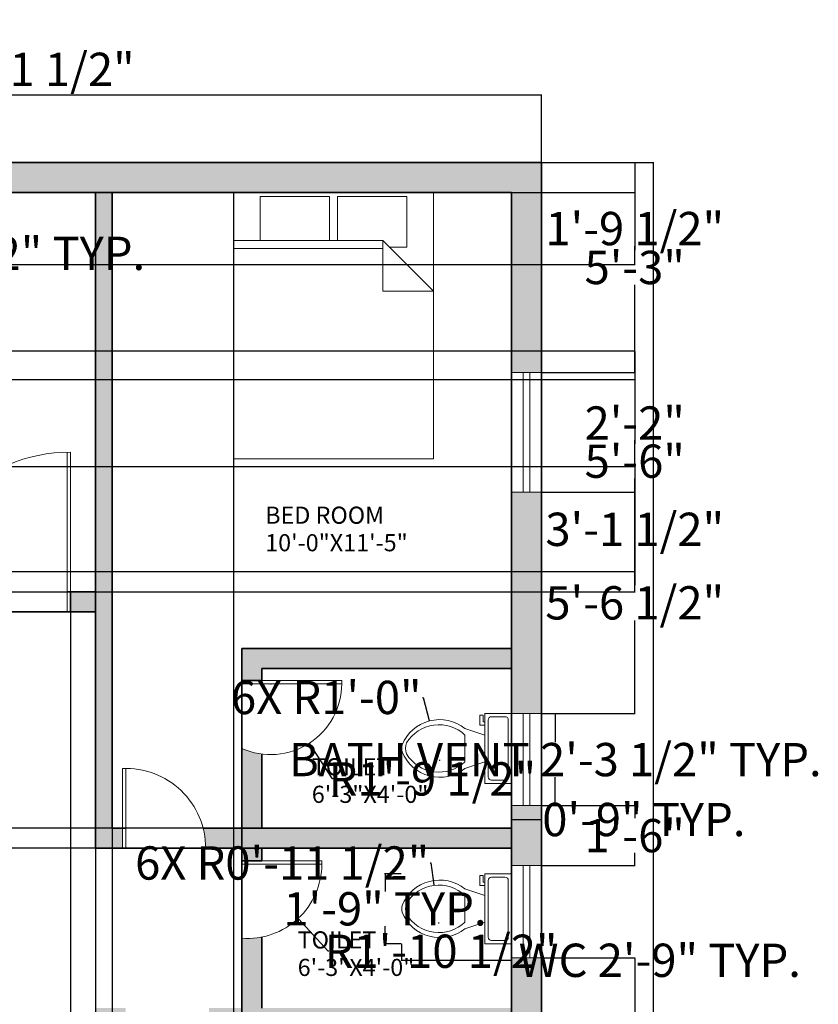
# Model space of a CAD drawing. Units: inches. Extents: x 2172 to 2712, y 1494 to 2108.
# Tile 3 of 3: x 2422 to 2662, y 1812 to 2108. Entities that reach past the tile are written whole.
import ezdxf

# ---------------------------------------------------------------- set-up
doc = ezdxf.new("R2010")
doc.units = ezdxf.units.IN
doc.header["$MEASUREMENT"] = 0
for name, color, linetype, lineweight in [('A-ANNO-DIMS', 2, 'Continuous', 18), ('A-AREA-IDEN', 7, 'Continuous', 18), ('A-DOOR', 3, 'Continuous', 18), ('A-FLOR-FIXT', 9, 'Continuous', 18), ('A-FURN', 8, 'Continuous', 18), ('A-GLAZ', 4, 'Continuous', 18), ('A-WALL', 7, 'Continuous', 35)]:
    doc.layers.add(name, color=color, linetype=linetype, lineweight=lineweight)
doc.layers.add('A-WALL-PATT', color=251, linetype='Continuous', lineweight=13, true_color=0x636466)
doc.styles.get("Standard").update_dxf_attribs({"font": 'arial.ttf'})
doc.dimstyles.get("Standard").update_dxf_attribs({"dimtxt": 10, "dimasz": 0.18, "dimexe": 0.18, "dimexo": 0.0625, "dimgap": 0.09, "dimtad": 0, "dimtih": 1, "dimtoh": 1, "dimdec": 0, "dimzin": 0, "dimdsep": 46, "dimlunit": 3, "dimtxsty": 'Standard', "dimcen": 0.09, "dimadec": 0, "dimazin": 0, "dimtfac": 1, "dimtdec": 0, "dimtofl": 0, "dimtmove": 0, "dimatfit": 3, "dimfxl": 1, "dimtolj": 1, "dimtzin": 0, "dimarcsym": 0})

# ---------------------------------------------------------------- blocks, each defined once
blk = doc.blocks.new('Toilet - top')
for p, q in [((9.5, -6), (9.5, -2)), ((-10, -8.5), (-8, -8.5)), ((-10, -9.5), (-10, -8.5)), ((-8, -8.5), (-8, -8)), ((-7, -8), (-7, -9.5)), ((-4, -8), (-6, -14)), ((4, -8), (6, -14)), ((-7, -9.5), (-10, -9.5)), ((4, -14), (-4, -14))]:
    blk.add_line(p, q)
blk.add_lwpolyline([(10.5, -8), (10.5, 0), (-10.5, 0), (-10.5, -8)], close=True)
for points in [[(-9.5, -2), (-9.5, -6)], [(8.5, -1), (-8.5, -1)], [(-8.5, -7), (8.5, -7)]]:
    blk.add_lwpolyline(points)
for centre, radius, start, end in [((-8.62, -1.88), 0.884, 81.8699, 188.1301), ((8.62, -1.88), 0.884, 351.8699, 98.1301), ((-8.62, -6.12), 0.884, 171.8699, 278.1301), ((8.62, -6.12), 0.884, 261.8699, 8.1301), ((3.52, -21.58), 12.17, 141.4691, 247.9714), ((4.2, -21.82), 11.33, 136.3677, 238.9468), ((-3.52, -21.58), 12.17, 292.0284, 38.5307), ((-4.2, -21.82), 11.33, 301.053, 43.6321), ((0, -27.88), 4, 245.7318, 294.2682), ((0, -29), 4, 254.8605, 285.1395)]:
    blk.add_arc(centre, radius, start, end)
blk = doc.blocks.new('Bed - Queen')
for p, q in [((0, -80.00003), (0, 0)), ((0, 0), (59.99999, 0)), ((59.99999, 0), (59.99999, -80.00003)), ((7.99999, -1.2), (28.79998, -1.2)), ((7.99999, -14.4), (7.99999, -1.2)), ((28.79998, -1.2), (28.79998, -14.4)), ((31.19999, -1.2), (51.99999, -1.2)), ((31.19999, -14.4), (31.19999, -1.2)), ((51.99999, -1.2), (51.99999, -16.4)), ((0, -14.4), (44.8, -14.4)), ((59.99999, -29.6), (44.8, -14.4)), ((44.8, -14.4), (44.8, -29.6)), ((44.8, -16.8), (0, -16.8)), ((51.99999, -16.4), (46.79936, -16.4)), ((44.8, -29.6), (59.99999, -29.6)), ((59.99999, -80.00003), (0, -80.00003))]:
    blk.add_line(p, q)
blk = doc.blocks.new('*D3')
at = {"layer": 'A-ANNO-DIMS', "color": 0, "lineweight": -2, "transparency": 16777216}
for p, q in [((2230.53, 2064.8), (2230.53, 2085.18)), ((2230.71, 2085), (2395.86, 2085)), ((2578.35, 2085), (2413.19, 2085)), ((2578.53, 2064.8), (2578.53, 2085.18))]:
    blk.add_line(p, q, dxfattribs=at)
at = {"layer": 'A-ANNO-DIMS', "color": 0, "transparency": 16777216}
for points in [[(2230.71, 2085.03), (2230.71, 2084.97), (2230.53, 2085)], [(2578.35, 2085.03), (2578.35, 2084.97), (2578.53, 2085)]]:
    blk.add_solid(points, dxfattribs=at)
at = {"layer": 'Defpoints', "color": 0, "transparency": 16777216}
for p in [(2578.53, 2085), (2230.53, 2064.74), (2578.53, 2064.74)]:
    blk.add_point(p, dxfattribs=at)
at = {"layer": 'A-ANNO-DIMS', "color": 0, "transparency": 16777216, "insert": (2404.53, 2085), "char_height": 10, "attachment_point": 5}
blk.add_mtext("\\A1;29'", dxfattribs=at)
blk = doc.blocks.new('*D4')
at = {"layer": 'A-ANNO-DIMS', "color": 0, "lineweight": -2, "transparency": 16777216}
for p, q in [((2578.59, 2064.74), (2612.28, 2064.74)), ((2612.1, 2064.56), (2612.1, 1805.83)), ((2612.1, 1536.92), (2612.1, 1795.65)), ((2578.59, 1536.74), (2612.28, 1536.74))]:
    blk.add_line(p, q, dxfattribs=at)
at = {"layer": 'A-ANNO-DIMS', "color": 0, "transparency": 16777216}
for points in [[(2612.07, 2064.56), (2612.13, 2064.56), (2612.1, 2064.74)], [(2612.07, 1536.92), (2612.13, 1536.92), (2612.1, 1536.74)]]:
    blk.add_solid(points, dxfattribs=at)
at = {"layer": 'Defpoints', "color": 0, "transparency": 16777216}
for p in [(2578.53, 2064.74), (2578.53, 1536.74), (2612.1, 1536.74)]:
    blk.add_point(p, dxfattribs=at)
at = {"layer": 'A-ANNO-DIMS', "color": 0, "transparency": 16777216, "insert": (2612.1, 1800.74), "char_height": 10, "attachment_point": 5}
blk.add_mtext("\\A1;44'", dxfattribs=at)
blk = doc.blocks.new('WIN-36IN')
for p, q in [((0, 36), (9, 36)), ((3.5, 36), (3.5, 0)), ((5.5, 36), (5.5, 0)), ((9, 0), (0, 0))]:
    blk.add_line(p, q)
blk = doc.blocks.new('WIN-BATH-VENT')
for p, q in [((0, 27.69), (9, 27.69)), ((3.5, 27.69), (3.5, 0)), ((5.5, 27.69), (5.5, 0)), ((0, 0), (9, 0))]:
    blk.add_line(p, q)
blk = doc.blocks.new('DOOR-SWING-48IN')
for p, q in [((47, 0), (47, 48)), ((48, 0), (48, 48))]:
    blk.add_line(p, q)
blk.add_arc((48, 0), 48, 90, 180)
blk = doc.blocks.new('*D11')
at = {"layer": 'A-ANNO-DIMS', "color": 0, "lineweight": -2, "transparency": 16777216}
for p, q in [((2578.59, 1899.23), (2582.86, 1899.23)), ((2582.68, 1899.05), (2582.68, 1890.65)), ((2582.68, 1871.72), (2582.68, 1880.12)), ((2578.59, 1871.54), (2582.86, 1871.54))]:
    blk.add_line(p, q, dxfattribs=at)
at = {"layer": 'A-ANNO-DIMS', "color": 0, "transparency": 16777216}
for points in [[(2582.65, 1899.05), (2582.71, 1899.05), (2582.68, 1899.23)], [(2582.65, 1871.72), (2582.71, 1871.72), (2582.68, 1871.54)]]:
    blk.add_solid(points, dxfattribs=at)
at = {"layer": 'Defpoints', "color": 0, "transparency": 16777216}
for p in [(2578.53, 1899.23), (2582.68, 1899.23), (2578.53, 1871.54)]:
    blk.add_point(p, dxfattribs=at)
at = {"layer": 'A-ANNO-DIMS', "color": 0, "transparency": 16777216, "insert": (2582.68, 1885.38), "char_height": 10, "attachment_point": 5}
blk.add_mtext('\\A1;BATH VENT 2\'-3 1/2" TYP.', dxfattribs=at)
blk = doc.blocks.new('*D12')
at = {"layer": 'A-ANNO-DIMS', "color": 0, "lineweight": -2, "transparency": 16777216}
for p, q in [((2569.53, 1871.47), (2569.53, 1867.2)), ((2578.53, 1871.47), (2578.53, 1867.2)), ((2569.71, 1867.38), (2578.35, 1867.38)), ((2578.53, 1867.38), (2578.71, 1867.38))]:
    blk.add_line(p, q, dxfattribs=at)
at = {"layer": 'A-ANNO-DIMS', "color": 0, "transparency": 16777216}
for points in [[(2569.71, 1867.41), (2569.71, 1867.35), (2569.53, 1867.38)], [(2578.35, 1867.41), (2578.35, 1867.35), (2578.53, 1867.38)]]:
    blk.add_solid(points, dxfattribs=at)
at = {"layer": 'Defpoints', "color": 0, "transparency": 16777216}
for p in [(2569.53, 1871.54), (2578.53, 1871.54), (2578.53, 1867.38)]:
    blk.add_point(p, dxfattribs=at)
at = {"layer": 'A-ANNO-DIMS', "color": 0, "transparency": 16777216, "insert": (2609.27, 1867.38), "char_height": 10, "attachment_point": 5}
blk.add_mtext('\\A1;0\'-9" TYP.', dxfattribs=at)
blk = doc.blocks.new('*D15')
at = {"layer": 'A-ANNO-DIMS', "color": 0, "lineweight": -2, "transparency": 16777216}
for p, q in [((2536.48, 1829.99), (2536.48, 1824.91)), ((2569.53, 1829.99), (2569.53, 1824.91)), ((2536.66, 1825.09), (2569.35, 1825.09)), ((2569.53, 1825.09), (2569.71, 1825.09))]:
    blk.add_line(p, q, dxfattribs=at)
at = {"layer": 'A-ANNO-DIMS', "color": 0, "transparency": 16777216}
for points in [[(2536.66, 1825.12), (2536.66, 1825.06), (2536.48, 1825.09)], [(2569.35, 1825.12), (2569.35, 1825.06), (2569.53, 1825.09)]]:
    blk.add_solid(points, dxfattribs=at)
at = {"layer": 'Defpoints', "color": 0, "transparency": 16777216}
for p in [(2536.48, 1830.05), (2569.53, 1830.05), (2569.53, 1825.09)]:
    blk.add_point(p, dxfattribs=at)
at = {"layer": 'A-ANNO-DIMS', "color": 0, "transparency": 16777216, "insert": (2614.06, 1825.09), "char_height": 10, "attachment_point": 5}
blk.add_mtext('\\A1;WC 2\'-9" TYP.', dxfattribs=at)
blk = doc.blocks.new('*D16')
at = {"layer": 'A-ANNO-DIMS', "color": 0, "lineweight": -2, "transparency": 16777216}
for p, q in [((2536.42, 1851.05), (2531.34, 1851.05)), ((2531.52, 1850.87), (2531.52, 1845.75)), ((2531.52, 1830.23), (2531.52, 1835.36)), ((2536.42, 1830.05), (2531.34, 1830.05))]:
    blk.add_line(p, q, dxfattribs=at)
at = {"layer": 'A-ANNO-DIMS', "color": 0, "transparency": 16777216}
for points in [[(2531.49, 1850.87), (2531.55, 1850.87), (2531.52, 1851.05)], [(2531.49, 1830.23), (2531.55, 1830.23), (2531.52, 1830.05)]]:
    blk.add_solid(points, dxfattribs=at)
at = {"layer": 'Defpoints', "color": 0, "transparency": 16777216}
for p in [(2536.48, 1851.05), (2531.52, 1830.05), (2536.48, 1830.05)]:
    blk.add_point(p, dxfattribs=at)
at = {"layer": 'A-ANNO-DIMS', "color": 0, "transparency": 16777216, "insert": (2531.52, 1840.55), "char_height": 10, "attachment_point": 5}
blk.add_mtext('\\A1;1\'-9" TYP.', dxfattribs=at)
blk = doc.blocks.new('*D19')
at = {"layer": 'A-ANNO-DIMS', "color": 0, "lineweight": -2, "transparency": 16777216}
for p, q in [((2301.42, 2039.44), (2301.42, 2037.28)), ((2315.03, 2039.44), (2315.03, 2037.28)), ((2301.6, 2037.46), (2314.85, 2037.46)), ((2315.03, 2037.46), (2315.21, 2037.46))]:
    blk.add_line(p, q, dxfattribs=at)
at = {"layer": 'A-ANNO-DIMS', "color": 0, "transparency": 16777216}
for points in [[(2301.6, 2037.49), (2301.6, 2037.43), (2301.42, 2037.46)], [(2314.85, 2037.49), (2314.85, 2037.43), (2315.03, 2037.46)]]:
    blk.add_solid(points, dxfattribs=at)
at = {"layer": 'Defpoints', "color": 0, "transparency": 16777216}
for p in [(2301.42, 2039.5), (2315.03, 2039.5), (2315.03, 2037.46)]:
    blk.add_point(p, dxfattribs=at)
at = {"layer": 'A-ANNO-DIMS', "color": 0, "transparency": 16777216, "insert": (2388.65, 2037.46), "char_height": 10, "attachment_point": 5}
blk.add_mtext('\\A1;BURNER 1\'-1 1/2" TYP.', dxfattribs=at)
blk = doc.blocks.new('*D24')
at = {"layer": 'A-ANNO-DIMS', "color": 0, "lineweight": -2, "transparency": 16777216}
for p, q in [((2578.59, 2064.74), (2606.71, 2064.74)), ((2606.53, 2064.56), (2606.53, 2038.42)), ((2606.53, 2001.89), (2606.53, 2028.02)), ((2578.59, 2001.71), (2606.71, 2001.71))]:
    blk.add_line(p, q, dxfattribs=at)
at = {"layer": 'A-ANNO-DIMS', "color": 0, "transparency": 16777216}
for points in [[(2606.5, 2064.56), (2606.56, 2064.56), (2606.53, 2064.74)], [(2606.5, 2001.89), (2606.56, 2001.89), (2606.53, 2001.71)]]:
    blk.add_solid(points, dxfattribs=at)
at = {"layer": 'Defpoints', "color": 0, "transparency": 16777216}
for p in [(2578.53, 2064.74), (2578.53, 2001.71), (2606.53, 2001.71)]:
    blk.add_point(p, dxfattribs=at)
at = {"layer": 'A-ANNO-DIMS', "color": 0, "transparency": 16777216, "insert": (2606.53, 2033.22), "char_height": 10, "attachment_point": 5}
blk.add_mtext('\\A1;5\'-3"', dxfattribs=at)
blk = doc.blocks.new('*D25')
at = {"layer": 'A-ANNO-DIMS', "color": 0, "lineweight": -2, "transparency": 16777216}
for p, q in [((2578.59, 1965.71), (2606.71, 1965.71)), ((2606.53, 1965.53), (2606.53, 1937.73)), ((2606.53, 1899.41), (2606.53, 1927.21)), ((2578.59, 1899.23), (2606.71, 1899.23))]:
    blk.add_line(p, q, dxfattribs=at)
at = {"layer": 'A-ANNO-DIMS', "color": 0, "transparency": 16777216}
for points in [[(2606.5, 1965.53), (2606.56, 1965.53), (2606.53, 1965.71)], [(2606.5, 1899.41), (2606.56, 1899.41), (2606.53, 1899.23)]]:
    blk.add_solid(points, dxfattribs=at)
at = {"layer": 'Defpoints', "color": 0, "transparency": 16777216}
for p in [(2578.53, 1965.71), (2578.53, 1899.23), (2606.53, 1899.23)]:
    blk.add_point(p, dxfattribs=at)
at = {"layer": 'A-ANNO-DIMS', "color": 0, "transparency": 16777216, "insert": (2606.53, 1932.47), "char_height": 10, "attachment_point": 5}
blk.add_mtext('\\A1;5\'-6 1/2"', dxfattribs=at)
blk = doc.blocks.new('*D26')
at = {"layer": 'A-ANNO-DIMS', "color": 0, "lineweight": -2, "transparency": 16777216}
for p, q in [((2578.59, 1871.54), (2606.71, 1871.54)), ((2606.53, 1871.36), (2606.53, 1867.74)), ((2606.53, 1853.72), (2606.53, 1857.34)), ((2578.59, 1853.54), (2606.71, 1853.54))]:
    blk.add_line(p, q, dxfattribs=at)
at = {"layer": 'A-ANNO-DIMS', "color": 0, "transparency": 16777216}
for points in [[(2606.5, 1871.36), (2606.56, 1871.36), (2606.53, 1871.54)], [(2606.5, 1853.72), (2606.56, 1853.72), (2606.53, 1853.54)]]:
    blk.add_solid(points, dxfattribs=at)
at = {"layer": 'Defpoints', "color": 0, "transparency": 16777216}
for p in [(2578.53, 1871.54), (2578.53, 1853.54), (2606.53, 1853.54)]:
    blk.add_point(p, dxfattribs=at)
at = {"layer": 'A-ANNO-DIMS', "color": 0, "transparency": 16777216, "insert": (2606.53, 1862.54), "char_height": 10, "attachment_point": 5}
blk.add_mtext('\\A1;1\'-6"', dxfattribs=at)
blk = doc.blocks.new('*D27')
at = {"layer": 'A-ANNO-DIMS', "color": 0, "lineweight": -2, "transparency": 16777216}
for p, q in [((2578.59, 1825.85), (2606.71, 1825.85)), ((2606.53, 1825.67), (2606.53, 1796.83)), ((2606.53, 1757.47), (2606.53, 1786.31)), ((2578.59, 1757.29), (2606.71, 1757.29))]:
    blk.add_line(p, q, dxfattribs=at)
at = {"layer": 'A-ANNO-DIMS', "color": 0, "transparency": 16777216}
for points in [[(2606.5, 1825.67), (2606.56, 1825.67), (2606.53, 1825.85)], [(2606.5, 1757.47), (2606.56, 1757.47), (2606.53, 1757.29)]]:
    blk.add_solid(points, dxfattribs=at)
at = {"layer": 'Defpoints', "color": 0, "transparency": 16777216}
for p in [(2578.53, 1825.85), (2578.53, 1757.29), (2606.53, 1757.29)]:
    blk.add_point(p, dxfattribs=at)
at = {"layer": 'A-ANNO-DIMS', "color": 0, "transparency": 16777216, "insert": (2606.53, 1791.57), "char_height": 10, "attachment_point": 5}
blk.add_mtext('\\A1;5\'-8 1/2"', dxfattribs=at)
blk = doc.blocks.new('*D32')
at = {"layer": 'A-ANNO-DIMS', "color": 0, "lineweight": -2, "transparency": 16777216}
for p, q in [((2391.23, 1545.8), (2391.23, 2092.92)), ((2391.41, 2092.74), (2404.56, 2092.74)), ((2404.74, 1545.8), (2404.74, 2092.92)), ((2404.74, 2092.74), (2404.92, 2092.74))]:
    blk.add_line(p, q, dxfattribs=at)
at = {"layer": 'A-ANNO-DIMS', "color": 0, "transparency": 16777216}
for points in [[(2391.41, 2092.77), (2391.41, 2092.71), (2391.23, 2092.74)], [(2404.56, 2092.77), (2404.56, 2092.71), (2404.74, 2092.74)]]:
    blk.add_solid(points, dxfattribs=at)
at = {"layer": 'Defpoints', "color": 0, "transparency": 16777216}
for p in [(2404.74, 2092.74), (2391.23, 1545.74), (2404.74, 1545.74)]:
    blk.add_point(p, dxfattribs=at)
at = {"layer": 'A-ANNO-DIMS', "color": 0, "transparency": 16777216, "insert": (2429.48, 2092.74), "char_height": 10, "attachment_point": 5}
blk.add_mtext('\\A1;1\'-1 1/2"', dxfattribs=at)
blk = doc.blocks.new('*D35')
at = {"layer": 'A-ANNO-DIMS', "color": 0, "lineweight": -2, "transparency": 16777216}
for p, q in [((2335.59, 2055.74), (2606.71, 2055.74)), ((2606.53, 2055.56), (2606.53, 2050.17)), ((2606.53, 2034.27), (2606.53, 2039.65)), ((2335.59, 2034.09), (2606.71, 2034.09))]:
    blk.add_line(p, q, dxfattribs=at)
at = {"layer": 'A-ANNO-DIMS', "color": 0, "transparency": 16777216}
for points in [[(2606.5, 2055.56), (2606.56, 2055.56), (2606.53, 2055.74)], [(2606.5, 2034.27), (2606.56, 2034.27), (2606.53, 2034.09)]]:
    blk.add_solid(points, dxfattribs=at)
at = {"layer": 'Defpoints', "color": 0, "transparency": 16777216}
for p in [(2335.53, 2055.74), (2335.53, 2034.09), (2606.53, 2034.09)]:
    blk.add_point(p, dxfattribs=at)
at = {"layer": 'A-ANNO-DIMS', "color": 0, "transparency": 16777216, "insert": (2606.53, 2044.91), "char_height": 10, "attachment_point": 5}
blk.add_mtext('\\A1;1\'-9 1/2"', dxfattribs=at)
blk = doc.blocks.new('*D37')
at = {"layer": 'A-ANNO-DIMS', "color": 0, "lineweight": -2, "transparency": 16777216}
for p, q in [((2258.5, 1999.6), (2606.71, 1999.6)), ((2606.53, 1999.42), (2606.53, 1991.6)), ((2606.53, 1973.56), (2606.53, 1981.38)), ((2258.5, 1973.38), (2606.71, 1973.38))]:
    blk.add_line(p, q, dxfattribs=at)
at = {"layer": 'A-ANNO-DIMS', "color": 0, "transparency": 16777216}
for points in [[(2606.5, 1999.42), (2606.56, 1999.42), (2606.53, 1999.6)], [(2606.5, 1973.56), (2606.56, 1973.56), (2606.53, 1973.38)]]:
    blk.add_solid(points, dxfattribs=at)
at = {"layer": 'Defpoints', "color": 0, "transparency": 16777216}
for p in [(2258.44, 1999.6), (2258.44, 1973.38), (2606.53, 1973.38)]:
    blk.add_point(p, dxfattribs=at)
at = {"layer": 'A-ANNO-DIMS', "color": 0, "transparency": 16777216, "insert": (2606.53, 1986.49), "char_height": 10, "attachment_point": 5}
blk.add_mtext('\\A1;2\'-2"', dxfattribs=at)
blk = doc.blocks.new('*D38')
at = {"layer": 'A-ANNO-DIMS', "color": 0, "lineweight": -2, "transparency": 16777216}
for p, q in [((2335.59, 2008.15), (2606.71, 2008.15)), ((2606.53, 2007.97), (2606.53, 1980.23)), ((2606.53, 1942.09), (2606.53, 1969.84)), ((2335.59, 1941.91), (2606.71, 1941.91))]:
    blk.add_line(p, q, dxfattribs=at)
at = {"layer": 'A-ANNO-DIMS', "color": 0, "transparency": 16777216}
for points in [[(2606.5, 2007.97), (2606.56, 2007.97), (2606.53, 2008.15)], [(2606.5, 1942.09), (2606.56, 1942.09), (2606.53, 1941.91)]]:
    blk.add_solid(points, dxfattribs=at)
at = {"layer": 'Defpoints', "color": 0, "transparency": 16777216}
for p in [(2335.53, 2008.15), (2335.53, 1941.91), (2606.53, 1941.91)]:
    blk.add_point(p, dxfattribs=at)
at = {"layer": 'A-ANNO-DIMS', "color": 0, "transparency": 16777216, "insert": (2606.53, 1975.03), "char_height": 10, "attachment_point": 5}
blk.add_mtext('\\A1;5\'-6"', dxfattribs=at)
blk = doc.blocks.new('*D41')
at = {"layer": 'A-ANNO-DIMS', "color": 0, "lineweight": -2, "transparency": 16777216}
for p, q in [((2437.05, 1929.68), (2437.05, 1508.56)), ((2444.53, 1929.68), (2444.53, 1508.56)), ((2437.23, 1508.74), (2444.35, 1508.74)), ((2444.53, 1508.74), (2444.71, 1508.74))]:
    blk.add_line(p, q, dxfattribs=at)
at = {"layer": 'A-ANNO-DIMS', "color": 0, "transparency": 16777216}
for points in [[(2437.23, 1508.77), (2437.23, 1508.71), (2437.05, 1508.74)], [(2444.35, 1508.77), (2444.35, 1508.71), (2444.53, 1508.74)]]:
    blk.add_solid(points, dxfattribs=at)
at = {"layer": 'Defpoints', "color": 0, "transparency": 16777216}
for p in [(2437.05, 1929.74), (2444.53, 1929.74), (2444.53, 1508.74)]:
    blk.add_point(p, dxfattribs=at)
at = {"layer": 'A-ANNO-DIMS', "color": 0, "transparency": 16777216, "insert": (2469.74, 1508.74), "char_height": 10, "attachment_point": 5}
blk.add_mtext('\\A1;0\'-7 1/2"', dxfattribs=at)
blk = doc.blocks.new('*D44')
at = {"layer": 'A-ANNO-DIMS', "color": 0, "lineweight": -2, "transparency": 16777216}
for p, q in [((2494.46, 1864.74), (2202.35, 1864.74)), ((2202.53, 1864.74), (2202.53, 1864.92)), ((2202.53, 1864.92), (2202.71, 1864.92)), ((2202.53, 1858.92), (2202.53, 1864.56)), ((2488.46, 1858.74), (2202.35, 1858.74))]:
    blk.add_line(p, q, dxfattribs=at)
at = {"layer": 'A-ANNO-DIMS', "color": 0, "transparency": 16777216}
for points in [[(2202.5, 1864.56), (2202.56, 1864.56), (2202.53, 1864.74)], [(2202.5, 1858.92), (2202.56, 1858.92), (2202.53, 1858.74)]]:
    blk.add_solid(points, dxfattribs=at)
at = {"layer": 'Defpoints', "color": 0, "transparency": 16777216}
for p in [(2202.53, 1864.74), (2494.53, 1864.74), (2488.53, 1858.74)]:
    blk.add_point(p, dxfattribs=at)
at = {"layer": 'A-ANNO-DIMS', "color": 0, "transparency": 16777216, "insert": (2216.09, 1864.92), "char_height": 10, "attachment_point": 5}
blk.add_mtext('\\A1;0\'-6"', dxfattribs=at)
blk = doc.blocks.new('*D45')
at = {"layer": 'A-ANNO-DIMS', "color": 0, "lineweight": -2, "transparency": 16777216}
for p, q in [((2258.5, 1973.38), (2606.71, 1973.38)), ((2606.53, 1973.2), (2606.53, 1959.83)), ((2606.53, 1935.92), (2606.53, 1949.3)), ((2262.05, 1935.74), (2606.71, 1935.74))]:
    blk.add_line(p, q, dxfattribs=at)
at = {"layer": 'A-ANNO-DIMS', "color": 0, "transparency": 16777216}
for points in [[(2606.5, 1973.2), (2606.56, 1973.2), (2606.53, 1973.38)], [(2606.5, 1935.92), (2606.56, 1935.92), (2606.53, 1935.74)]]:
    blk.add_solid(points, dxfattribs=at)
at = {"layer": 'Defpoints', "color": 0, "transparency": 16777216}
for p in [(2258.44, 1973.38), (2261.99, 1935.74), (2606.53, 1935.74)]:
    blk.add_point(p, dxfattribs=at)
at = {"layer": 'A-ANNO-DIMS', "color": 0, "transparency": 16777216, "insert": (2606.53, 1954.56), "char_height": 10, "attachment_point": 5}
blk.add_mtext('\\A1;3\'-1 1/2"', dxfattribs=at)
blk = doc.blocks.new('*D47')
at = {"layer": 'A-ANNO-DIMS', "color": 0, "lineweight": -2, "transparency": 16777216}
for p, q in [((2449.53, 2055.68), (2449.53, 1508.56)), ((2486.06, 2055.68), (2486.06, 1508.56)), ((2449.71, 1508.74), (2485.88, 1508.74)), ((2486.06, 1508.74), (2486.24, 1508.74))]:
    blk.add_line(p, q, dxfattribs=at)
at = {"layer": 'A-ANNO-DIMS', "color": 0, "transparency": 16777216}
for points in [[(2449.71, 1508.77), (2449.71, 1508.71), (2449.53, 1508.74)], [(2485.88, 1508.77), (2485.88, 1508.71), (2486.06, 1508.74)]]:
    blk.add_solid(points, dxfattribs=at)
at = {"layer": 'Defpoints', "color": 0, "transparency": 16777216}
for p in [(2449.53, 2055.74), (2486.06, 2055.74), (2486.06, 1508.74)]:
    blk.add_point(p, dxfattribs=at)
at = {"layer": 'A-ANNO-DIMS', "color": 0, "transparency": 16777216, "insert": (2511.27, 1508.74), "char_height": 10, "attachment_point": 5}
blk.add_mtext('\\A1;3\'-0 1/2"', dxfattribs=at)
blk = doc.blocks.new('*D51')
at = {"layer": 'A-ANNO-DIMS', "color": 0, "lineweight": -2, "transparency": 16777216}
for p, q in [((2490.11, 1854), (2490.29, 1854)), ((2490.2, 1853.91), (2490.2, 1854.09)), ((2514.49, 1827.81), (2505.51, 1837.5)), ((2514.67, 1827.81), (2514.49, 1827.81))]:
    blk.add_line(p, q, dxfattribs=at)
at = {"layer": 'A-ANNO-DIMS', "color": 0, "transparency": 16777216}
blk.add_solid([(2505.53, 1837.52), (2505.48, 1837.48), (2505.38, 1837.64)], dxfattribs=at)
at = {"layer": 'Defpoints', "color": 0, "transparency": 16777216}
for p in [(2490.2, 1854), (2505.38, 1837.64)]:
    blk.add_point(p, dxfattribs=at)
at = {"layer": 'A-ANNO-DIMS', "color": 0, "transparency": 16777216, "insert": (2548.37, 1827.81), "char_height": 10, "attachment_point": 5}
blk.add_mtext('\\A1;R1\'-10 1/2"', dxfattribs=at)
blk = doc.blocks.new('*D52')
at = {"layer": 'A-ANNO-DIMS', "color": 0, "lineweight": -2, "transparency": 16777216}
for p, q in [((2497.14, 1908.18), (2497.32, 1908.18)), ((2497.23, 1908.09), (2497.23, 1908.27)), ((2515.76, 1879.58), (2508.91, 1890.15)), ((2515.94, 1879.58), (2515.76, 1879.58))]:
    blk.add_line(p, q, dxfattribs=at)
at = {"layer": 'A-ANNO-DIMS', "color": 0, "transparency": 16777216}
blk.add_solid([(2508.93, 1890.17), (2508.88, 1890.14), (2508.81, 1890.3)], dxfattribs=at)
at = {"layer": 'Defpoints', "color": 0, "transparency": 16777216}
for p in [(2497.23, 1908.18), (2508.81, 1890.3)]:
    blk.add_point(p, dxfattribs=at)
at = {"layer": 'A-ANNO-DIMS', "color": 0, "transparency": 16777216, "insert": (2545.75, 1879.58), "char_height": 10, "attachment_point": 5}
blk.add_mtext('\\A1;R1\'-9 1/2"', dxfattribs=at)
blk = doc.blocks.new('*D53')
at = {"layer": 'A-ANNO-DIMS', "color": 0, "lineweight": -2, "transparency": 16777216}
for p, q in [((2542.82, 1904.05), (2543, 1904.05)), ((2543, 1904.05), (2544.81, 1897.16)), ((2547.85, 1885.22), (2548.03, 1885.22)), ((2547.94, 1885.13), (2547.94, 1885.31))]:
    blk.add_line(p, q, dxfattribs=at)
at = {"layer": 'A-ANNO-DIMS', "color": 0, "transparency": 16777216}
blk.add_solid([(2544.84, 1897.17), (2544.78, 1897.16), (2544.85, 1896.99)], dxfattribs=at)
at = {"layer": 'Defpoints', "color": 0, "transparency": 16777216}
for p in [(2544.85, 1896.99), (2547.94, 1885.22)]:
    blk.add_point(p, dxfattribs=at)
at = {"layer": 'A-ANNO-DIMS', "color": 0, "transparency": 16777216, "insert": (2513.88, 1904.05), "char_height": 10, "attachment_point": 5}
blk.add_mtext('\\A1;6X R1\'-0"', dxfattribs=at)
blk = doc.blocks.new('*D54')
at = {"layer": 'A-ANNO-DIMS', "color": 0, "lineweight": -2, "transparency": 16777216}
for p, q in [((2545.11, 1854.32), (2545.29, 1854.32)), ((2545.29, 1854.32), (2546.17, 1847.76)), ((2547.62, 1836.35), (2547.8, 1836.35)), ((2547.71, 1836.26), (2547.71, 1836.44))]:
    blk.add_line(p, q, dxfattribs=at)
at = {"layer": 'A-ANNO-DIMS', "color": 0, "transparency": 16777216}
blk.add_solid([(2546.2, 1847.76), (2546.14, 1847.75), (2546.2, 1847.58)], dxfattribs=at)
at = {"layer": 'Defpoints', "color": 0, "transparency": 16777216}
for p in [(2546.2, 1847.58), (2547.71, 1836.35)]:
    blk.add_point(p, dxfattribs=at)
at = {"layer": 'A-ANNO-DIMS', "color": 0, "transparency": 16777216, "insert": (2500.64, 1854.32), "char_height": 10, "attachment_point": 5}
blk.add_mtext('\\A1;6X R0\'-11 1/2"', dxfattribs=at)

msp = doc.modelspace()

# ---------------------------------------------------------------- hatches: boundary and pattern name
at = {"layer": 'A-WALL-PATT'}
h = msp.add_hatch(color=256, dxfattribs=at)
h.dxf.hatch_style = 1
h.paths.add_polyline_path([(2239.53, 1774.79), (2230.53, 1774.79), (2230.53, 1536.74), (2245.63, 1536.74), (2245.63, 1541.24), (2239.53, 1541.24)])
h.paths.add_polyline_path([(2569.53, 1545.74), (2379.53, 1545.74), (2379.53, 1536.74), (2569.53, 1536.74)])
h.paths.add_polyline_path([(2379.53, 1541.24), (2344.11, 1541.24), (2344.11, 1536.74), (2379.3, 1536.74)])
h.paths.add_polyline_path([(2578.53, 1561.68), (2569.53, 1561.68), (2569.53, 1536.74), (2578.53, 1536.74)])
h.paths.add_polyline_path([(2578.53, 1628.83), (2569.53, 1628.83), (2569.53, 1618.74), (2569.53, 1597.68), (2578.53, 1597.68)])
h.paths.add_polyline_path([(2578.53, 1721.29), (2569.53, 1721.29), (2569.53, 1672.74), (2569.53, 1656.53), (2578.53, 1656.53)])
h.paths.add_polyline_path([(2569.53, 1672.74), (2479.6, 1672.74, -0.062096), (2478.72, 1666.74), (2569.53, 1666.74)], flags=17)
h.paths.add_polyline_path([(2569.53, 1618.74), (2449.53, 1618.74), (2449.53, 1666.74), (2454.6, 1666.74), (2454.6, 1672.74), (2449.53, 1672.74), (2449.53, 1804.74), (2453.65, 1804.74), (2453.65, 1810.74), (2444.53, 1810.74), (2444.53, 1739.74), (2436.58, 1739.74), (2436.58, 1730.74), (2444.53, 1730.74), (2444.53, 1612.74), (2569.53, 1612.74)])
h.paths.add_polyline_path([(2384.53, 1730.74), (2379.53, 1730.74), (2379.53, 1612.74), (2384.53, 1612.74)])
h.paths.add_polyline_path([(2389.43, 1739.74), (2239.53, 1739.74), (2239.53, 1730.74), (2388.58, 1730.74, -0.047189)])
h.paths.add_polyline_path([(2569.53, 1810.74), (2494.53, 1810.74), (2494.53, 1832.1, -0.067617), (2488.53, 1831.74), (2488.53, 1830), (2488.53, 1804.74), (2569.53, 1804.74)])
h.paths.add_polyline_path([(2488.53, 1810.74), (2478.65, 1810.74, -0.063254), (2477.89, 1804.74), (2488.53, 1804.74)])
h.paths.add_polyline_path([(2569.53, 1864.74), (2488.53, 1864.74), (2488.53, 1858.74), (2569.53, 1858.74)])
h.paths.add_polyline_path([(2494.53, 1858.74), (2488.53, 1858.74), (2488.53, 1855), (2494.53, 1855)])
h.paths.add_polyline_path([(2494.53, 1887.05, -0.073561), (2488.53, 1888.74), (2488.53, 1885.18), (2488.53, 1879.18), (2488.53, 1864.74), (2494.53, 1864.74)])
h.paths.add_polyline_path([(2488.53, 1864.74), (2476.91, 1864.74, -0.063254), (2477.67, 1858.74), (2488.53, 1858.74)])
h.paths.add_polyline_path([(2449.53, 1918.74), (2449.53, 2055.74), (2444.53, 2055.74), (2444.53, 1912.74), (2444.53, 1858.74), (2449.53, 1858.74), (2452.67, 1858.74), (2452.67, 1864.74), (2449.53, 1864.74)])
h.paths.add_polyline_path([(2578.53, 1965.71), (2569.53, 1965.71), (2569.53, 1918.74), (2569.53, 1899.23), (2578.53, 1899.23)])
h.paths.add_polyline_path([(2578.53, 1825.85), (2569.53, 1825.85), (2569.53, 1757.29), (2578.53, 1757.29)])
h.paths.add_polyline_path([(2578.53, 1871.54), (2569.53, 1871.54), (2569.53, 1864.74), (2569.53, 1853.54), (2578.53, 1853.54)])
h.paths.add_polyline_path([(2239.53, 1884.82), (2230.53, 1884.82), (2230.53, 1810.79), (2239.53, 1810.79)])
h.paths.add_polyline_path([(2239.53, 1968.53), (2230.53, 1968.53), (2230.53, 1920.82), (2239.53, 1920.82), (2239.53, 1929.74)])
h.paths.add_polyline_path([(2389.42, 1935.74), (2340.53, 1935.74), (2340.53, 1941.91), (2335.53, 1941.91), (2335.53, 1935.74), (2239.53, 1935.74), (2239.53, 1929.74), (2340.53, 1929.74), (2389.05, 1929.74, -0.031342)])
h.paths.add_polyline_path([(2239.53, 2055.74), (2569.53, 2055.74), (2569.53, 2001.71), (2578.53, 2001.71), (2578.53, 2064.74), (2230.53, 2064.74), (2230.53, 2004.53), (2239.53, 2004.53)])
h.paths.add_polyline_path([(2340.53, 2055.74), (2335.53, 2055.74), (2335.53, 2008.15), (2340.53, 2008.15)], flags=17)
h.paths.add_polyline_path([(2444.53, 1935.74), (2437.05, 1935.74), (2437.05, 1929.74), (2444.53, 1929.74)])
h.paths.add_polyline_path([(2569.53, 1918.74), (2488.53, 1918.74), (2488.53, 1909.18), (2494.53, 1909.18), (2494.53, 1912.74), (2569.53, 1912.74)])

# ---------------------------------------------------------------- linework, layer by layer
at = {"layer": 'A-DOOR'}
for p, q in [((2488.53, 1909.18), (2518.53, 1909.18)), ((2488.53, 1909.18), (2488.53, 1879.18)), ((2488.53, 1909.18), (2488.53, 1885.18)), ((2518.53, 1908.18), (2488.53, 1908.18)), ((2518.53, 1909.18), (2518.53, 1908.18)), ((2452.67, 1858.74), (2452.67, 1882.74)), ((2453.67, 1882.74), (2453.67, 1858.74)), ((2488.53, 1855), (2512.53, 1855)), ((2512.53, 1855), (2512.53, 1854)), ((2512.53, 1854), (2488.53, 1854)), ((2488.53, 1854), (2488.53, 1830))]:
    msp.add_line(p, q, dxfattribs=at)
for centre, radius, start, end in [((2497.23, 1908.18), 21.3, 245.8792, 0), ((2453.67, 1858.74), 24, 0, 92.388), ((2490.2, 1854), 22.33, 265.6975, 360)]:
    msp.add_arc(centre, radius, start, end, dxfattribs=at)
at = {"layer": 'A-WALL'}
for p, q in [((2230.53, 2064.74), (2578.53, 2064.74)), ((2578.53, 2064.74), (2578.53, 1536.74)), ((2239.53, 2055.74), (2569.53, 2055.74)), ((2443.53, 2055.74), (2443.53, 2055.74)), ((2444.53, 1912.74), (2444.53, 2055.74)), ((2449.53, 1918.74), (2449.53, 2055.74)), ((2569.53, 2055.74), (2569.53, 1536.74)), ((2569.53, 2055.74), (2569.53, 1918.74)), ((2444.53, 1935.74), (2436.05, 1935.74)), ((2437.05, 1929.74), (2437.05, 1935.74)), ((2444.53, 1929.74), (2335.53, 1929.74)), ((2449.53, 1864.74), (2449.53, 1918.74)), ((2569.53, 1918.74), (2488.53, 1918.74)), ((2488.53, 1858.74), (2488.53, 1918.74)), ((2444.53, 1912.74), (2444.53, 1858.74)), ((2569.53, 1912.74), (2494.53, 1912.74)), ((2494.53, 1908.18), (2494.53, 1912.74)), ((2569.53, 1912.74), (2569.53, 1864.74)), ((2494.53, 1909.18), (2488.53, 1909.18)), ((2494.53, 1864.74), (2494.53, 1887.05)), ((2453.67, 1864.74), (2449.53, 1864.74)), ((2569.53, 1864.74), (2476.91, 1864.74)), ((2444.53, 1858.74), (2444.53, 1858.74)), ((2444.53, 1858.74), (2449.53, 1858.74)), ((2488.53, 1858.74), (2449.53, 1858.74)), ((2569.53, 1858.74), (2488.53, 1858.74)), ((2488.53, 1804.74), (2488.53, 1858.74)), ((2494.53, 1855), (2494.53, 1858.74)), ((2569.53, 1858.74), (2569.53, 1810.74)), ((2488.53, 1855), (2494.53, 1855)), ((2494.53, 1810.74), (2494.53, 1832.1))]:
    msp.add_line(p, q, dxfattribs=at)

# ---------------------------------------------------------------- block references
at = {"layer": 'A-DOOR'}
msp.add_blockref('DOOR-SWING-48IN', (2389.05, 1929.74), dxfattribs=at)
at = {"layer": 'A-FLOR-FIXT', "rotation": 270}
for p in [(2569.53, 1888.74), (2569.53, 1840.55)]:
    msp.add_blockref('Toilet - top', p, dxfattribs=at)
at = {"layer": 'A-FURN'}
msp.add_blockref('Bed - Queen', (2486.06, 2055.74), dxfattribs=at)
at = {"layer": 'A-GLAZ'}
for name, p in [('WIN-36IN', (2569.53, 1965.71)), ('WIN-BATH-VENT', (2569.53, 1871.54)), ('WIN-BATH-VENT', (2569.53, 1825.85))]:
    msp.add_blockref(name, p, dxfattribs=at)

# ---------------------------------------------------------------- texts
at = {"layer": 'A-AREA-IDEN'}
for s, height, p in [('BED ROOM ', 5.144, (2495.53, 1956.23)), ('10\'-0"X11\'-5"', 5.1443, (2495.53, 1947.96)), ('TOILET', 5.144, (2509.53, 1880.64)), ('6\'-3"X4\'-0"', 5.1443, (2509.53, 1872.38)), ('TOILET', 5.144, (2505.29, 1828.64)), ('6\'-3"X4\'-0"', 5.1443, (2505.29, 1820.38))]:
    msp.add_text(s, height=height, dxfattribs=at).set_placement(p)

# ---------------------------------------------------------------- dimensions: what is measured, and where the dimension line sits
at = {"layer": 'A-ANNO-DIMS'}
for base, p1, p2, override, picture, middle in [((2404.74, 2092.74), (2391.23, 1545.74), (2404.74, 1545.74), {"dimdec": 1, "dimlfac": 1, "dimrnd": 0, "dimzin": 1, "dimdsep": 46, "dimlunit": 4, "dimfrac": 2}, '*D32', (2429.48, 2092.74)), ((2578.53, 2085), (2230.53, 2064.74), (2578.53, 2064.74), {"dimclrd": 0, "dimclre": 0, "dimclrt": 0}, '*D3', (2404.53, 2085)), ((2486.06, 1508.74), (2449.53, 2055.74), (2486.06, 2055.74), {"dimdec": 1, "dimlfac": 1, "dimrnd": 0, "dimzin": 1, "dimdsep": 46, "dimlunit": 4, "dimfrac": 2}, '*D47', (2511.27, 1508.74)), ((2444.53, 1508.74), (2437.05, 1929.74), (2444.53, 1929.74), {"dimdec": 1, "dimlfac": 1, "dimrnd": 0, "dimzin": 1, "dimdsep": 46, "dimlunit": 4, "dimfrac": 2}, '*D41', (2469.74, 1508.74))]:
    dim = msp.add_linear_dim(base=base, p1=p1, p2=p2, dimstyle='Standard', override=override, dxfattribs=at)
    dim.commit()
    dim.dimension.update_dxf_attribs({"geometry": picture, "text_midpoint": middle})
for base, p1, p2, text, picture, middle in [((2315.03, 2037.46), (2301.42, 2039.5), (2315.03, 2039.5), 'BURNER <> TYP.', '*D19', (2388.65, 2037.46)), ((2578.53, 1867.38), (2569.53, 1871.54), (2578.53, 1871.54), '<> TYP.', '*D12', (2609.27, 1867.38)), ((2569.5253, 1825.0942), (2536.479, 1830.0512), (2569.5253, 1830.0512), 'WC <> TYP.', '*D15', (2614.0552, 1825.0942))]:
    dim = msp.add_linear_dim(base=base, p1=p1, p2=p2, text=text, dimstyle='Standard', override={"dimdec": 1, "dimlfac": 1, "dimrnd": 0, "dimzin": 1, "dimdsep": 46, "dimlunit": 4, "dimfrac": 2}, dxfattribs=at)
    dim.commit()
    dim.dimension.update_dxf_attribs({"geometry": picture, "text_midpoint": middle})
for base, p1, p2, override, picture, middle in [((2612.1, 1536.74), (2578.53, 2064.74), (2578.53, 1536.74), {"dimclrd": 0, "dimclre": 0, "dimclrt": 0}, '*D4', (2612.1, 1800.74)), ((2606.53, 2001.71), (2578.53, 2064.74), (2578.53, 2001.71), {"dimdec": 1, "dimlfac": 1, "dimrnd": 0, "dimzin": 1, "dimdsep": 46, "dimlunit": 4, "dimfrac": 2}, '*D24', (2606.53, 2033.22)), ((2606.5253, 2034.0872), (2335.5253, 2055.7407), (2335.5253, 2034.0872), {"dimdec": 1, "dimlfac": 1, "dimrnd": 0, "dimzin": 1, "dimdsep": 46, "dimlunit": 4, "dimfrac": 2}, '*D35', (2606.5253, 2044.914)), ((2606.53, 1941.91), (2335.53, 2008.15), (2335.53, 1941.91), {"dimdec": 1, "dimlfac": 1, "dimrnd": 0, "dimzin": 1, "dimdsep": 46, "dimlunit": 4, "dimfrac": 2}, '*D38', (2606.53, 1975.03)), ((2606.53, 1973.38), (2258.44, 1999.6), (2258.44, 1973.38), {"dimdec": 1, "dimlfac": 1, "dimrnd": 0, "dimzin": 1, "dimdsep": 46, "dimlunit": 4, "dimfrac": 2}, '*D37', (2606.53, 1986.49)), ((2606.53, 1935.74), (2258.44, 1973.38), (2261.99, 1935.74), {"dimdec": 1, "dimlfac": 1, "dimrnd": 0, "dimzin": 1, "dimdsep": 46, "dimlunit": 4, "dimfrac": 2}, '*D45', (2606.53, 1954.56)), ((2606.53, 1899.23), (2578.53, 1965.71), (2578.53, 1899.23), {"dimdec": 1, "dimlfac": 1, "dimrnd": 0, "dimzin": 1, "dimdsep": 46, "dimlunit": 4, "dimfrac": 2}, '*D25', (2606.53, 1932.47)), ((2202.53, 1864.74), (2488.53, 1858.74), (2494.53, 1864.74), {"dimdec": 1, "dimlfac": 1, "dimrnd": 0, "dimzin": 1, "dimdsep": 46, "dimlunit": 4, "dimfrac": 2}, '*D44', (2216.09, 1864.92)), ((2606.53, 1853.54), (2578.53, 1871.54), (2578.53, 1853.54), {"dimdec": 1, "dimlfac": 1, "dimrnd": 0, "dimzin": 1, "dimdsep": 46, "dimlunit": 4, "dimfrac": 2}, '*D26', (2606.53, 1862.54)), ((2606.53, 1757.29), (2578.53, 1825.85), (2578.53, 1757.29), {"dimdec": 1, "dimlfac": 1, "dimrnd": 0, "dimzin": 1, "dimdsep": 46, "dimlunit": 4, "dimfrac": 2}, '*D27', (2606.53, 1791.57))]:
    dim = msp.add_linear_dim(base=base, p1=p1, p2=p2, angle=90, dimstyle='Standard', override=override, dxfattribs=at)
    dim.commit()
    dim.dimension.update_dxf_attribs({"geometry": picture, "text_midpoint": middle})
for base, p1, p2, angle, text, picture, middle in [((2582.68, 1899.23), (2578.53, 1871.54), (2578.53, 1899.23), 90, 'BATH VENT <> TYP.', '*D11', (2582.68, 1885.38)), ((2531.52, 1830.05), (2536.48, 1851.05), (2536.48, 1830.05), 270, '<> TYP.', '*D16', (2531.52, 1840.55))]:
    dim = msp.add_linear_dim(base=base, p1=p1, p2=p2, angle=angle, text=text, dimstyle='Standard', override={"dimdec": 1, "dimlfac": 1, "dimrnd": 0, "dimzin": 1, "dimdsep": 46, "dimlunit": 4, "dimfrac": 2}, dxfattribs=at)
    dim.commit()
    dim.dimension.update_dxf_attribs({"geometry": picture, "text_midpoint": middle})
for center, mpoint, picture, middle in [((2547.94, 1885.22), (2544.85, 1896.99), '*D53', (2513.88, 1904.05)), ((2547.71, 1836.35), (2546.2, 1847.58), '*D54', (2500.64, 1854.32))]:
    dim = msp.add_radius_dim(center=center, mpoint=mpoint, text='6X <>', dimstyle='Standard', override={"dimdec": 1, "dimlfac": 1, "dimrnd": 0, "dimzin": 1, "dimdsep": 46, "dimlunit": 4, "dimfrac": 2}, dxfattribs=at)
    dim.commit()
    dim.dimension.update_dxf_attribs({"geometry": picture, "text_midpoint": middle, "dimtype": 164})
for center, mpoint, picture, middle in [((2497.23, 1908.18), (2508.81, 1890.3), '*D52', (2545.75, 1879.58)), ((2490.2, 1854), (2505.38, 1837.64), '*D51', (2548.37, 1827.81))]:
    dim = msp.add_radius_dim(center=center, mpoint=mpoint, dimstyle='Standard', override={"dimdec": 1, "dimlfac": 1, "dimrnd": 0, "dimzin": 1, "dimdsep": 46, "dimlunit": 4, "dimfrac": 2}, dxfattribs=at)
    dim.commit()
    dim.dimension.update_dxf_attribs({"geometry": picture, "text_midpoint": middle, "dimtype": 164})

doc.saveas('drawing.dxf')
